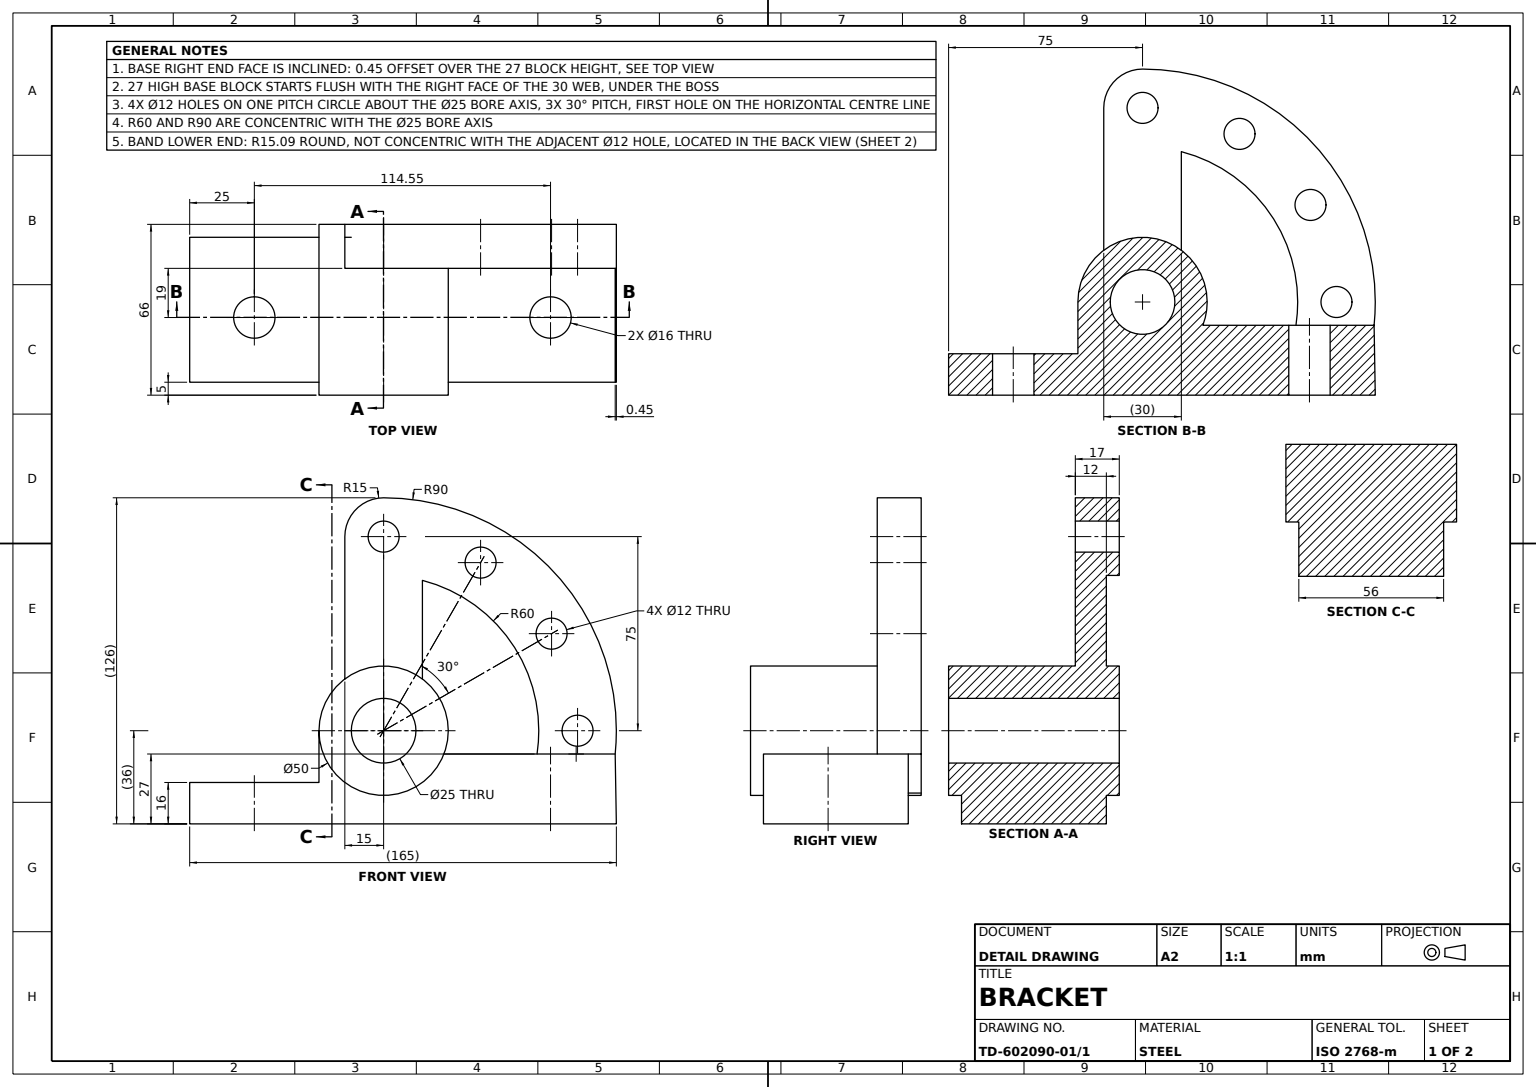
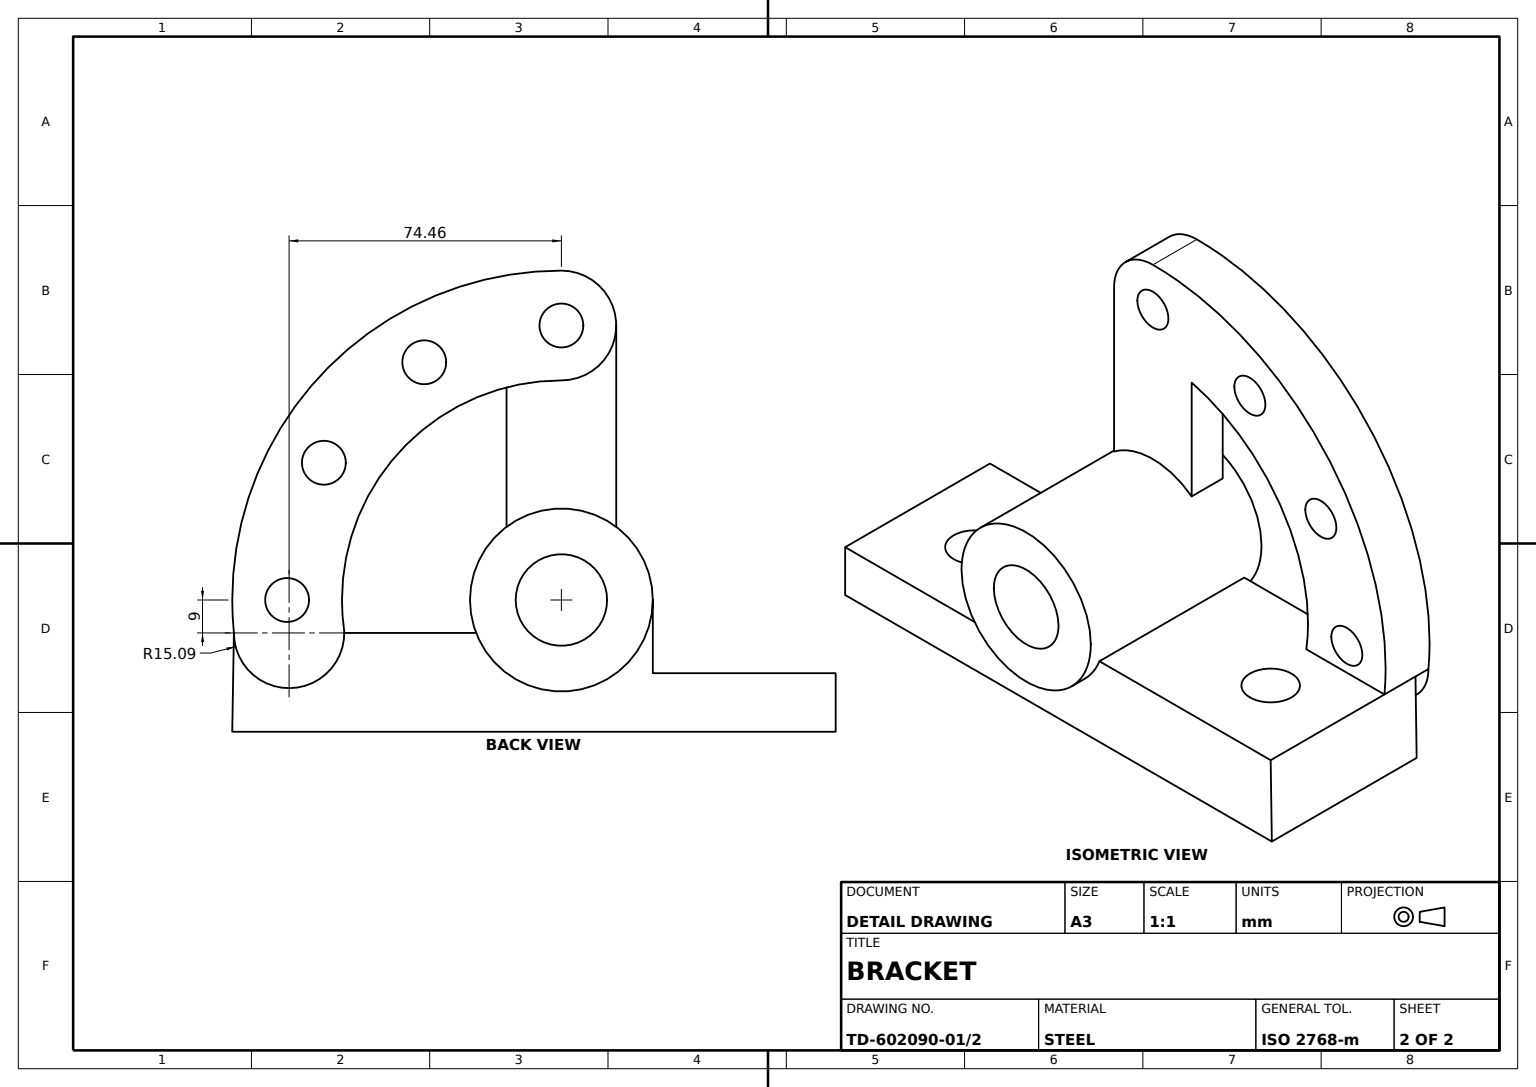
from build123d import *

# Parameters (mm, degrees)
STEPPED_BASE_BLOCK_DEPTH           = 61
STEPPED_BASE_BLOCK_DEPTH_BACK      = 5
BRACKET_PROFILE_SKETCH_R           = 25
BRACKET_PROFILE_SKETCH_R_2         = 12.5
BEARING_BOSS_DEPTH                 = 56
QUADRANT_MOUNTING_PLATE_DEPTH      = 12
QUADRANT_MOUNTING_PLATE_DEPTH_BACK = 5
SKETCH1_9_R                        = 6
UPRIGHT_WEB_DEPTH                  = 12
BASE_HOLES_SKETCH_R                = 8
BASE_THROUGH_HOLES_DEPTH           = 98


with BuildPart() as part:
    # Bracket Profile Sketch → Stepped Base Block (new, two sides: drawn at the far end of the back side and taken through both)
    with BuildSketch(Plane.XY.offset(-STEPPED_BASE_BLOCK_DEPTH_BACK)):
        with Locations((75, 36)):
            Circle(BRACKET_PROFILE_SKETCH_R)
        with Locations((75, 36)):
            Circle(BRACKET_PROFILE_SKETCH_R_2, mode=Mode.SUBTRACT)
    extrude(amount=STEPPED_BASE_BLOCK_DEPTH + STEPPED_BASE_BLOCK_DEPTH_BACK)

    # Sketch1_5 → Bearing Boss (add)
    with BuildSketch(Plane.XY):
        with BuildLine():
            Line((0, 16), (0, 0))
            Line((0, 0), (75, 0))
            Line((75, 0), (165, 0))
            Line((165, 0), (164.54886934, 27))
            ThreePointArc((164.54886934, 27), (149.458041876, 11.909172536), (134.367214412, 27))
            Line((134.367214412, 27), (134.3211598, 27))
            Line((134.3211598, 27), (98.323807579, 27))
            ThreePointArc((98.323807579, 27), (70.422620263, 11.422620263), (50, 36))
            Line((50, 36), (50, 16))
            Line((50, 16), (0, 16))
        make_face()
        with BuildLine():
            ThreePointArc((134.367214412, 27), (149.458041876, 11.909172536), (164.54886934, 27))
            Line((164.54886934, 27), (134.367214412, 27))
        make_face()
    extrude(amount=BEARING_BOSS_DEPTH)

    # Sketch1_9 → Quadrant Mounting Plate (add, two sides: drawn at the far end of the back side and taken through both)
    # profile 1 of 2: a face of its own
    with BuildSketch(Plane.XY.offset(-QUADRANT_MOUNTING_PLATE_DEPTH_BACK)):
        with BuildLine():
            Line((134.367214412, 27), (164.54886934, 27))
            ThreePointArc((164.54886934, 27), (141.745786384, 96.373835392), (75, 126))
            ThreePointArc((75, 126), (64.393398282, 121.606601718), (60, 111))
            ThreePointArc((60, 111), (64.393398282, 100.393398282), (75, 96))
            ThreePointArc((75, 96), (82.560257549, 95.521781776), (90, 94.094750193))
            ThreePointArc((90, 94.094750193), (124.13637209, 70.432788703), (134.725771353, 30.270057917))
            ThreePointArc((134.725771353, 30.270057917), (134.566433501, 28.8), (134.370917994, 27.334315001))
            ThreePointArc((134.370917994, 27.334315001), (134.368140336, 27.167167757), (134.367214412, 27))
        make_face()
        with Locations((150, 36)):
            Circle(SKETCH1_9_R, mode=Mode.SUBTRACT)
        with Locations((75, 111)):
            Circle(SKETCH1_9_R, mode=Mode.SUBTRACT)
        with Locations((139.951905284, 73.5)):
            Circle(SKETCH1_9_R, mode=Mode.SUBTRACT)
        with Locations((112.5, 100.951905284)):
            Circle(SKETCH1_9_R, mode=Mode.SUBTRACT)
    # profile 2 of 2: a face of its own
    with BuildSketch(Plane.XY.offset(-QUADRANT_MOUNTING_PLATE_DEPTH_BACK)):
        with BuildLine():
            ThreePointArc((134.367214412, 27), (149.458041876, 11.909172536), (164.54886934, 27))
            Line((164.54886934, 27), (134.367214412, 27))
        make_face()
    extrude(amount=QUADRANT_MOUNTING_PLATE_DEPTH + QUADRANT_MOUNTING_PLATE_DEPTH_BACK)

    # Sketch1_10 → Upright Web (add)
    with BuildSketch(Plane.XY):
        with BuildLine():
            Line((60, 61), (60, 56))
            ThreePointArc((60, 56), (75, 61), (90, 56))
            Line((90, 56), (90, 61))
            Line((90, 61), (90, 94.094750193))
            ThreePointArc((90, 94.094750193), (82.560257549, 95.521781776), (75, 96))
            ThreePointArc((75, 96), (64.393398282, 100.393398282), (60, 111))
            Line((60, 111), (60, 96))
            Line((60, 96), (60, 61))
        make_face()
    extrude(amount=UPRIGHT_WEB_DEPTH)

    # Base Holes Sketch → Base Through Holes (cut)
    with BuildSketch(Plane(origin=(0, 0, 0), x_dir=(1, 0, 0), z_dir=(0, 1, 0))):
        with Locations(Location((25, -31, 0), (0, 0, 90))):
            Circle(BASE_HOLES_SKETCH_R)
        with Locations(Location((139.54886934, -31, 0), (0, 0, 270))):
            Circle(BASE_HOLES_SKETCH_R)
    extrude(amount=BASE_THROUGH_HOLES_DEPTH, mode=Mode.SUBTRACT)


solid = part.part
